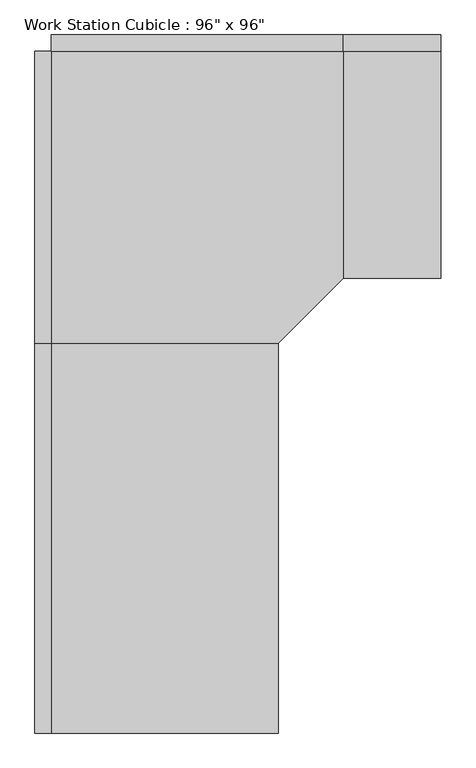
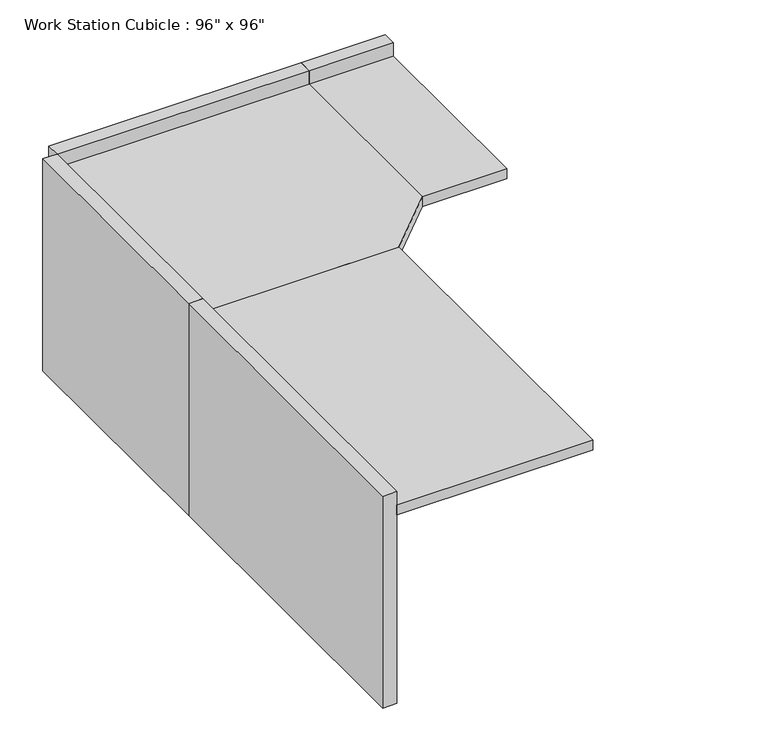
"""IFC4 building model written with IfcOpenShell, lengths in millimetres: furniture geometry."""

from ifc_helpers import new_model, si_unit, frame, origin, origin_with_axes, place, context, project, spatial, polyline, outline, extrude, source, transform, mapped, element, save


def furniture_25b31cd6(model_context):
    return source(origin(), model_context, "Body", "SweptSolid", [
        extrude(outline(polyline([(-80.9317522, -545.8230076), (833.4682478, -545.8230076), (833.4682478, -1257.0230076), (630.2682478, -1460.2230076), (-80.9317522, -1460.2230076), (-80.9317522, -545.8230076)])), frame((0.0, 0.0, 723.9), z_axis=(0.0, 0.0, 1.0), x_axis=(1.0, 0.0, 0.0)), (0.0, 0.0, 1.0), 38.1),
        extrude(outline(polyline([(630.2682478, -2679.4230076), (-80.9317522, -2679.4230076), (-80.9317522, -1460.2230076), (630.2682478, -1460.2230076), (630.2682478, -2679.4230076)])), frame((0.0, 0.0, 723.9), z_axis=(0.0, 0.0, 1.0), x_axis=(1.0, 0.0, 0.0)), (0.0, 0.0, 1.0), 38.1),
        extrude(outline(polyline([(1138.2682478, -1257.0230076), (833.4682478, -1257.0230076), (833.4682478, -545.8230076), (1138.2682478, -545.8230076), (1138.2682478, -1257.0230076)])), frame((0.0, 0.0, 723.9), z_axis=(0.0, 0.0, 1.0), x_axis=(1.0, 0.0, 0.0)), (0.0, 0.0, 1.0), 38.1),
        extrude(outline(polyline([(1138.2682478, -545.8230076), (833.4682478, -545.8230076), (833.4682478, -495.0230076), (1138.2682478, -495.0230076), (1138.2682478, -545.8230076)])), origin_with_axes(), (0.0, 0.0, 1.0), 812.8),
        extrude(outline(polyline([(833.4682478, -545.8230076), (-80.9317522, -545.8230076), (-80.9317522, -495.0230076), (833.4682478, -495.0230076), (833.4682478, -545.8230076)])), origin_with_axes(), (0.0, 0.0, 1.0), 812.8),
        extrude(outline(polyline([(-80.9317522, -1460.2230076), (-131.7317522, -1460.2230076), (-131.7317522, -545.8230076), (-80.9317522, -545.8230076), (-80.9317522, -1460.2230076)])), origin_with_axes(), (0.0, 0.0, 1.0), 812.8),
        extrude(outline(polyline([(-80.9317522, -2679.4230076), (-131.7317522, -2679.4230076), (-131.7317522, -1460.2230076), (-80.9317522, -1460.2230076), (-80.9317522, -2679.4230076)])), origin_with_axes(), (0.0, 0.0, 1.0), 812.8),
    ])


if __name__ == "__main__":
    model = new_model("IFC4")
    model_context = context("Model", 3, world=origin())
    ifc_project = project(units=[si_unit("LENGTHUNIT", "METRE", prefix="MILLI")], contexts=[model_context])
    site = spatial("IfcSite", under=ifc_project)
    building = spatial("IfcBuilding", under=site)
    placement = place(None, origin())
    furniture_shape = furniture_25b31cd6(model_context)
    element("IfcFurniture", 1, ObjectType="Work Station Cubicle : 96\" x 96\"", at=placement, inside=building, context=model_context, shape_type="MappedRepresentation", body=[
        mapped(furniture_shape, transform((0.0, 0.0, 0.0), x_axis=(1.0, 0.0, 0.0), y_axis=(0.0, 1.0, 0.0), z_axis=(0.0, 0.0, 1.0))),
    ])
    save(model, "model.ifc")

# Revit data of these elements
# Type "Work Station Cubicle : 96\" x 96\""
#   Assembly Code = "E2020"
#   Desktop Height = 2' - 6"
#   Desktop1 Width = 2' - 4"
#   Desktop2 Width = 2' - 4"
#   Panel Height = 2' - 8"
#   Panel1 Length = 4' - 0"
#   Panel2 Length = 1' - 0"
#   Cube Panel Material = Textile - Light Gray
#   Work Top Material = Laminate, Ivory, Matte
#   Default Elevation = 0
# Element 1 (IfcFurniture, "Work Station Cubicle : 96\" x 96\"")
#   Materials on its faces: "Textile - Light Gray", "Laminate, Ivory, Matte"
# Materials
#   "Textile - Light Gray": class "Fabric", colour RGB 204 204 204, transparency 0
#   "Laminate, Ivory, Matte": class "Plastic", colour RGB 247 247 239, transparency 0, Description = "Plastic Laminate - Ivory, Matte", Cost = 0
